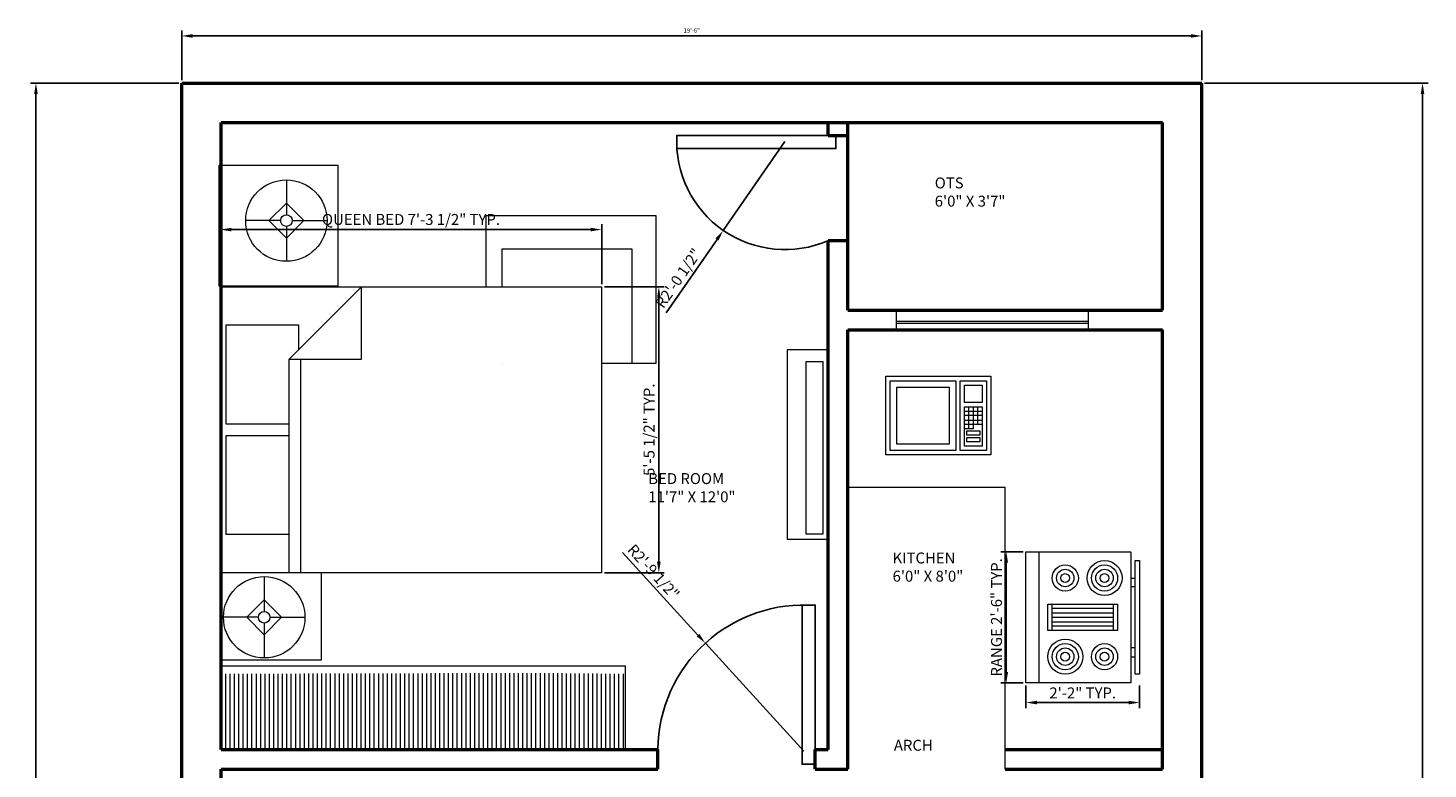
# Model space of a CAD drawing. Units: inches. Extents: x 210 to 950, y 0 to 561.
# Tile 3 of 5: x 228 to 548, y 382 to 551. Entities that reach past the tile are written whole.
import ezdxf

# ---------------------------------------------------------------- set-up
doc = ezdxf.new("R2010")
doc.units = ezdxf.units.IN
for name, color, linetype, lineweight in [('A-ANNO-DIMS', 2, 'Continuous', 18), ('A-ANNO-TEXT', 7, 'Continuous', 18), ('A-AREA-IDEN', 7, 'Continuous', 18), ('A-DOOR', 4, 'Continuous', 25), ('A-EQPM', 8, 'Continuous', 18), ('A-FLOR-CASE', 8, 'Continuous', 20), ('A-FURN', 8, 'Continuous', 18), ('A-FURN-PATT', 9, 'Continuous', 13), ('A-GLAZ', 4, 'Continuous', 20), ('A-WALL', 7, 'Continuous', 50)]:
    doc.layers.add(name, color=color, linetype=linetype, lineweight=lineweight)
doc.styles.get("Standard").update_dxf_attribs({"font": 'arial.ttf'})
doc.dimstyles.new('ISO-25', dxfattribs={"dimtxt": 2.5, "dimasz": 2.5, "dimexe": 1.25, "dimexo": 0.625, "dimtad": 1, "dimtxsty": 'Standard', "dimcen": 2.5, "dimadec": 0, "dimazin": 0, "dimtfac": 1, "dimtmove": 0, "dimatfit": 3, "dimfxl": 1, "dimarcsym": 0})

# ---------------------------------------------------------------- blocks, each defined once
blk = doc.blocks.new('Bed - Queen')
for p, q in [((0, -80.00003), (0, 0)), ((0, 0), (59.99999, 0)), ((59.99999, 0), (59.99999, -80.00003)), ((7.99999, -1.2), (28.79998, -1.2)), ((7.99999, -14.4), (7.99999, -1.2)), ((28.79998, -1.2), (28.79998, -14.4)), ((31.19999, -1.2), (51.99999, -1.2)), ((31.19999, -14.4), (31.19999, -1.2)), ((51.99999, -1.2), (51.99999, -16.4)), ((0, -14.4), (44.8, -14.4)), ((59.99999, -29.6), (44.8, -14.4)), ((44.8, -14.4), (44.8, -29.6)), ((44.8, -16.8), (0, -16.8)), ((51.99999, -16.4), (46.79936, -16.4)), ((44.8, -29.6), (59.99999, -29.6)), ((59.99999, -80.00003), (0, -80.00003))]:
    blk.add_line(p, q)
blk = doc.blocks.new('Lamp - Table')
for p, q in [((0, 7), (0, 1)), ((0, 3), (-3, 0)), ((3, 0), (0, 3)), ((-1, 0), (-7, 0)), ((-3, 0), (0, -3)), ((0, -3), (3, 0)), ((1, 0), (7, 0)), ((0, -1), (0, -7))]:
    blk.add_line(p, q)
for radius in [7, 1]:
    blk.add_circle((0, 0), radius)
blk = doc.blocks.new('Range-Oven - 30 in top')
for p, q in [((0, -3), (30, -3)), ((12, -6), (18, -6)), ((13, -20), (13, -6)), ((14, -6), (14, -20)), ((15, -20), (15, -6)), ((16, -6), (16, -20)), ((17, -20), (17, -6)), ((18, -20), (12, -20)), ((6, -24), (6, -25)), ((8, -25), (8, -24)), ((22, -25), (22, -24)), ((24, -24), (24, -25))]:
    blk.add_line(p, q)
for points in [[(0, -24), (0, 0), (30, 0), (30, -24)], [(12, -21), (12, -5), (18, -5), (18, -21)], [(2, -26), (2, -25), (28, -25), (28, -26)]]:
    blk.add_lwpolyline(points, close=True)
for centre, radius in [((6, -9), 4), ((6, -9), 3), ((24, -9), 3), ((6, -9), 2), ((6, -9), 1), ((24, -9), 2), ((24, -9), 1), ((6, -18), 3), ((6, -18), 2), ((24, -18), 4), ((24, -18), 3), ((24, -18), 2), ((6, -18), 1), ((24, -18), 1)]:
    blk.add_circle(centre, radius)
blk = doc.blocks.new('Microwave')
for p, q in [((18, 10), (22, 10)), ((19, 7), (19, 11)), ((20, 11), (20, 7)), ((21, 7), (21, 11)), ((22, 9), (18, 9)), ((18, 8), (22, 8)), ((22, 7), (18, 7)), ((19, 6), (19, 7)), ((20, 7), (20, 6)), ((20, 6), (18, 6))]:
    blk.add_line(p, q)
for points in [[(0, 0), (0, 18), (24, 18), (24, 0)], [(1, 1), (1, 17), (16, 17), (16, 1)], [(17, 1), (17, 17), (23, 17), (23, 1)], [(2.5, 2.5), (2.5, 15.5), (14.5, 15.5), (14.5, 2.5)], [(18, 12), (18, 16), (22, 16), (22, 12)], [(18, 2), (18, 11), (22, 11), (22, 2)], [(18.5, 4.5), (18.5, 5.5), (21.5, 5.5), (21.5, 4.5)], [(18.5, 3), (18.5, 4), (21.5, 4), (21.5, 3)]]:
    blk.add_lwpolyline(points, close=True)
blk = doc.blocks.new('*D14')
at = {"layer": 'A-ANNO-DIMS', "color": 0, "lineweight": -2, "transparency": 16777216}
for p, q in [((262.91, 539.13), (262.91, 550.53)), ((265.41, 549.28), (493.91, 549.28)), ((496.41, 539.13), (496.41, 550.53))]:
    blk.add_line(p, q, dxfattribs=at)
at = {"layer": 'A-ANNO-DIMS', "color": 0, "transparency": 16777216}
for points in [[(265.41, 549.7), (265.41, 548.87), (262.91, 549.28)], [(493.91, 549.7), (493.91, 548.87), (496.41, 549.28)]]:
    blk.add_solid(points, dxfattribs=at)
at = {"layer": 'Defpoints', "color": 0, "transparency": 16777216}
for p in [(496.41, 549.28), (262.91, 538.5), (496.41, 538.5)]:
    blk.add_point(p, dxfattribs=at)
at = {"layer": 'A-ANNO-DIMS', "color": 0, "transparency": 16777216, "insert": (379.66, 550.42), "char_height": 1, "attachment_point": 5}
blk.add_mtext('19\'-6"', dxfattribs=at)
blk = doc.blocks.new('*D15')
at = {"layer": 'A-ANNO-DIMS', "color": 0, "lineweight": -2, "transparency": 16777216}
for p, q in [((262.29, 538.5), (228.3, 538.5)), ((229.55, 61), (229.55, 536)), ((262.29, 58.5), (228.3, 58.5))]:
    blk.add_line(p, q, dxfattribs=at)
at = {"layer": 'A-ANNO-DIMS', "color": 0, "transparency": 16777216}
for points in [[(229.13, 536), (229.96, 536), (229.55, 538.5)], [(229.13, 61), (229.96, 61), (229.55, 58.5)]]:
    blk.add_solid(points, dxfattribs=at)
at = {"layer": 'Defpoints', "color": 0, "transparency": 16777216}
for p in [(229.55, 538.5), (262.91, 538.5), (262.91, 58.5)]:
    blk.add_point(p, dxfattribs=at)
at = {"layer": 'A-ANNO-DIMS', "color": 0, "transparency": 16777216, "insert": (228.41, 298.5), "char_height": 1, "attachment_point": 5, "rotation": 90}
blk.add_mtext("40'", dxfattribs=at)
blk = doc.blocks.new('*D16')
at = {"layer": 'A-ANNO-DIMS', "color": 0, "lineweight": -2, "transparency": 16777216}
for p, q in [((497.04, 538.5), (548.19, 538.5)), ((546.94, 57), (546.94, 536)), ((497.04, 54.5), (548.19, 54.5))]:
    blk.add_line(p, q, dxfattribs=at)
at = {"layer": 'A-ANNO-DIMS', "color": 0, "transparency": 16777216}
for points in [[(546.52, 536), (547.35, 536), (546.94, 538.5)], [(546.52, 57), (547.35, 57), (546.94, 54.5)]]:
    blk.add_solid(points, dxfattribs=at)
at = {"layer": 'Defpoints', "color": 0, "transparency": 16777216}
for p in [(496.41, 538.5), (546.94, 538.5), (496.41, 54.5)]:
    blk.add_point(p, dxfattribs=at)
at = {"layer": 'A-ANNO-DIMS', "color": 0, "transparency": 16777216, "insert": (545.8, 296.5), "char_height": 1, "attachment_point": 5, "rotation": 90}
blk.add_mtext('40\'-4"', dxfattribs=at)
blk = doc.blocks.new('DOOR-LEAF-36IN')
blk.add_lwpolyline([(0, 0), (0, -2.99), (-36.41, -2.99), (-36.41, 0)], close=True)
blk = doc.blocks.new('*D30')
at = {"layer": 'A-ANNO-DIMS', "color": 0, "lineweight": -2, "transparency": 16777216}
for p, q in [((271.77, 492.5), (271.77, 506.21)), ((356.54, 504.96), (274.27, 504.96)), ((359.04, 492.5), (359.04, 506.21))]:
    blk.add_line(p, q, dxfattribs=at)
at = {"layer": 'A-ANNO-DIMS', "color": 0, "transparency": 16777216}
for points in [[(274.27, 505.38), (274.27, 504.55), (271.77, 504.96)], [(356.54, 505.38), (356.54, 504.55), (359.04, 504.96)]]:
    blk.add_solid(points, dxfattribs=at)
at = {"layer": 'Defpoints', "color": 0, "transparency": 16777216}
for p in [(271.77, 504.96), (271.77, 491.87), (359.04, 491.87)]:
    blk.add_point(p, dxfattribs=at)
at = {"layer": 'A-ANNO-DIMS', "color": 0, "transparency": 16777216, "insert": (315.4, 506.96), "char_height": 2.5, "attachment_point": 5}
blk.add_mtext('QUEEN BED 7\'-3 1/2" TYP.', dxfattribs=at)
blk = doc.blocks.new('*D31')
at = {"layer": 'A-ANNO-DIMS', "color": 0, "lineweight": -2, "transparency": 16777216}
for p, q in [((359.66, 491.87), (373.38, 491.87)), ((372.13, 428.92), (372.13, 489.37)), ((359.66, 426.42), (373.38, 426.42))]:
    blk.add_line(p, q, dxfattribs=at)
at = {"layer": 'A-ANNO-DIMS', "color": 0, "transparency": 16777216}
for points in [[(371.71, 489.37), (372.54, 489.37), (372.13, 491.87)], [(371.71, 428.92), (372.54, 428.92), (372.13, 426.42)]]:
    blk.add_solid(points, dxfattribs=at)
at = {"layer": 'Defpoints', "color": 0, "transparency": 16777216}
for p in [(359.04, 491.87), (372.13, 491.87), (359.04, 426.42)]:
    blk.add_point(p, dxfattribs=at)
at = {"layer": 'A-ANNO-DIMS', "color": 0, "transparency": 16777216, "insert": (370.21, 459.15), "char_height": 2.5, "attachment_point": 5, "rotation": 90}
blk.add_mtext('5\'-5 1/2" TYP.', dxfattribs=at)
blk = doc.blocks.new('*D36')
at = {"layer": 'A-ANNO-DIMS', "color": 0, "lineweight": -2, "transparency": 16777216}
for p, q in [((455.53, 431.21), (450.4, 431.21)), ((451.65, 403.71), (451.65, 428.71)), ((455.53, 401.21), (450.4, 401.21))]:
    blk.add_line(p, q, dxfattribs=at)
at = {"layer": 'A-ANNO-DIMS', "color": 0, "transparency": 16777216}
for points in [[(451.24, 428.71), (452.07, 428.71), (451.65, 431.21)], [(451.24, 403.71), (452.07, 403.71), (451.65, 401.21)]]:
    blk.add_solid(points, dxfattribs=at)
at = {"layer": 'Defpoints', "color": 0, "transparency": 16777216}
for p in [(451.65, 431.21), (456.15, 431.21), (456.15, 401.21)]:
    blk.add_point(p, dxfattribs=at)
at = {"layer": 'A-ANNO-DIMS', "color": 0, "transparency": 16777216, "insert": (449.74, 416.21), "char_height": 2.5, "attachment_point": 5, "rotation": 90}
blk.add_mtext('RANGE 2\'-6" TYP.', dxfattribs=at)
blk = doc.blocks.new('*D37')
at = {"layer": 'A-ANNO-DIMS', "color": 0, "lineweight": -2, "transparency": 16777216}
for p, q in [((456.15, 400.58), (456.15, 395.46)), ((482.15, 400.58), (482.15, 395.46)), ((479.65, 396.71), (458.65, 396.71))]:
    blk.add_line(p, q, dxfattribs=at)
at = {"layer": 'A-ANNO-DIMS', "color": 0, "transparency": 16777216}
for points in [[(458.65, 397.13), (458.65, 396.29), (456.15, 396.71)], [(479.65, 397.13), (479.65, 396.29), (482.15, 396.71)]]:
    blk.add_solid(points, dxfattribs=at)
at = {"layer": 'Defpoints', "color": 0, "transparency": 16777216}
for p in [(456.15, 401.21), (482.15, 401.21), (456.15, 396.71)]:
    blk.add_point(p, dxfattribs=at)
at = {"layer": 'A-ANNO-DIMS', "color": 0, "transparency": 16777216, "insert": (469.15, 398.59), "char_height": 2.5, "attachment_point": 5}
blk.add_mtext('2\'-2" TYP.', dxfattribs=at)
blk = doc.blocks.new('*D53')
at = {"layer": 'A-ANNO-DIMS', "color": 0, "lineweight": -2, "transparency": 16777216}
for p, q in [((363.83, 431.06), (381.09, 412.15)), ((405.29, 385.62), (382.77, 410.3))]:
    blk.add_line(p, q, dxfattribs=at)
at = {"layer": 'A-ANNO-DIMS', "color": 0, "transparency": 16777216}
blk.add_solid([(381.4, 412.43), (380.78, 411.87), (382.77, 410.3)], dxfattribs=at)
at = {"layer": 'Defpoints', "color": 0, "transparency": 16777216}
for p in [(382.77, 410.3), (405.29, 385.62)]:
    blk.add_point(p, dxfattribs=at)
at = {"layer": 'A-ANNO-DIMS', "color": 0, "transparency": 16777216, "insert": (370.68, 426.4), "char_height": 2.5, "attachment_point": 5, "rotation": 312.3709}
blk.add_mtext('R2\'-9 1/2"', dxfattribs=at)
blk = doc.blocks.new('*D54')
at = {"layer": 'A-ANNO-DIMS', "color": 0, "lineweight": -2, "transparency": 16777216}
for p, q in [((400.96, 525.12), (386.87, 504.77)), ((373.83, 485.94), (385.45, 502.72))]:
    blk.add_line(p, q, dxfattribs=at)
at = {"layer": 'A-ANNO-DIMS', "color": 0, "transparency": 16777216}
blk.add_solid([(385.1, 502.96), (385.79, 502.48), (386.87, 504.77)], dxfattribs=at)
at = {"layer": 'Defpoints', "color": 0, "transparency": 16777216}
for p in [(400.96, 525.12), (386.87, 504.77)]:
    blk.add_point(p, dxfattribs=at)
at = {"layer": 'A-ANNO-DIMS', "color": 0, "transparency": 16777216, "insert": (376.84, 493.66), "char_height": 2.5, "attachment_point": 5, "rotation": 55.2977}
blk.add_mtext('R2\'-0 1/2"', dxfattribs=at)

msp = doc.modelspace()

# ---------------------------------------------------------------- hatches: boundary and pattern name
at = {"layer": 'A-FURN-PATT'}
h = msp.add_hatch(dxfattribs=at)
h.set_pattern_fill('ANSI31', color=256, scale=0.314961, angle=45, style=0)
h.paths.add_polyline_path([(271.97, 403.27), (271.97, 386.23), (297.62, 386.09), (322.62, 386.09), (364.47, 386.23), (364.47, 403.27), (348.68, 403.41), (323.68, 403.41)])

# ---------------------------------------------------------------- linework, layer by layer
at = {"layer": 'A-DOOR'}
for centre, radius, start, end in [((400.96, 525.12), 24.75, 176.8495, 293.746), ((405.29, 385.62), 33.41, 85.4748, 179.2678)]:
    msp.add_arc(centre, radius, start, end, dxfattribs=at)
at = {"layer": 'A-FLOR-CASE'}
for p in [(415.41, 446), (451.41, 381.5)]:
    msp.add_line(p, (451.41, 446), dxfattribs=at)
msp.add_lwpolyline([(271.86, 386.06), (364.51, 386.06), (364.51, 405.03), (271.86, 405.03)], close=True, dxfattribs=at)
at = {"layer": 'A-FURN'}
for points in [[(271.48, 519.7), (298.62, 519.7), (298.62, 492), (271.48, 492)], [(410.86, 477.41), (401.51, 477.41), (401.51, 434.14), (410.86, 434.14)], [(409.73, 474.7), (405.8, 474.7), (405.8, 435.33), (409.73, 435.33)], [(271.87, 426.46), (294.85, 426.46), (294.85, 406.39), (271.87, 406.39)]]:
    msp.add_lwpolyline(points, close=True, dxfattribs=at)
for points in [[(332.57, 491.87), (332.57, 508.16), (371.47, 508.16), (371.47, 474.33), (359.04, 474.33)], [(336.27, 491.87), (336.27, 500.53), (365.95, 500.53), (365.95, 474.28), (359.04, 474.28)], [(336.27, 474.28), (336.27, 474.33)]]:
    msp.add_lwpolyline(points, dxfattribs=at)
at = {"layer": 'A-GLAZ'}
for p, q in [((426.49, 482), (426.49, 486.5)), ((426.49, 486.5), (470.39, 486.5)), ((426.49, 484), (470.39, 484)), ((470.39, 486.5), (470.39, 482)), ((470.39, 483.5), (426.49, 483.5))]:
    msp.add_line(p, q, dxfattribs=at)
at = {"layer": 'A-WALL'}
for p, q in [((262.91, 54.5), (262.91, 538.5)), ((262.91, 538.5), (496.41, 538.5)), ((496.41, 54.5), (496.41, 538.5)), ((271.91, 529.5), (410.91, 529.5)), ((271.91, 386), (271.91, 529.5)), ((410.91, 529.5), (487.41, 529.5)), ((410.91, 526.5), (410.91, 529.5)), ((415.41, 526.5), (415.41, 529.5)), ((487.41, 486.5), (487.41, 529.5)), ((487.41, 486.5), (487.41, 529.5)), ((410.91, 526.5), (415.41, 526.5)), ((415.41, 486.5), (415.41, 526.5)), ((410.91, 386), (410.91, 502.5)), ((410.91, 502.5), (415.41, 502.5)), ((415.41, 486.5), (487.41, 486.5)), ((415.41, 381.5), (415.41, 482)), ((415.41, 482), (487.41, 482)), ((487.41, 381.5), (487.41, 482)), ((487.41, 386), (487.41, 482)), ((271.91, 386), (371.91, 386)), ((371.91, 381.5), (371.91, 386)), ((407.91, 381.5), (407.91, 386)), ((407.91, 386), (410.91, 386)), ((451.41, 386), (487.41, 386)), ((271.91, 381.5), (371.91, 381.5)), ((271.91, 249.5), (271.91, 381.5)), ((407.91, 381.5), (415.41, 381.5)), ((451.41, 381.5), (487.41, 381.5))]:
    msp.add_line(p, q, dxfattribs=at)

# ---------------------------------------------------------------- block references
at = {"layer": 'A-DOOR'}
msp.add_blockref('DOOR-LEAF-36IN', (412.67, 526.5), dxfattribs=at)
at = {"layer": 'A-DOOR', "rotation": 270}
msp.add_blockref('DOOR-LEAF-36IN', (407.92, 382.6), dxfattribs=at)
at = {"layer": 'A-EQPM'}
msp.add_blockref('Microwave', (424.11, 453.38), dxfattribs=at)
at = {"layer": 'A-EQPM', "rotation": 90}
msp.add_blockref('Range-Oven - 30 in top', (456.15, 401.21), dxfattribs=at)
at = {"layer": 'A-FURN', "xscale": 1.330786106251803, "yscale": 1.330786106251803, "zscale": 1.330786106251803}
for p in [(286.87, 507.02), (281.79, 416.23)]:
    msp.add_blockref('Lamp - Table', p, dxfattribs=at)
at = {"layer": 'A-FURN', "xscale": 1.090825566177695, "yscale": 1.090825566177695, "zscale": 1.090825566177695, "rotation": 90}
msp.add_blockref('Bed - Queen', (271.77, 426.42), dxfattribs=at)

# ---------------------------------------------------------------- texts
at = {"layer": 'A-ANNO-TEXT', "insert": (425.93, 388.18), "char_height": 2.5, "attachment_point": 1}
msp.add_mtext_dynamic_manual_height_columns('ARCH', width=6.915, gutter_width=12.5, heights=[0], dxfattribs=at)
at = {"layer": 'A-AREA-IDEN', "char_height": 2.5, "attachment_point": 1}
for s, width, insert in [('OTS\\P6\'0" X 3\'7"', 23.4882, (435.28, 516.89)), ('BED ROOM\\P11\'7" X 12\'0"', 30.419, (369.71, 449.22)), ('KITCHEN\\P\\pxt5;6\'0" X 8\'0"', 25.4662, (425.63, 431.05))]:
    msp.add_mtext_dynamic_manual_height_columns(s, width=width, gutter_width=12.5, heights=[0], dxfattribs=dict(at, insert=insert))

# ---------------------------------------------------------------- dimensions: what is measured, and where the dimension line sits
at = {"layer": 'A-ANNO-DIMS'}
dim = msp.add_linear_dim(base=(496.41085496, 549.28267643), p1=(262.91085496, 538.50240855), p2=(496.41085496, 538.50240855), dimstyle='ISO-25', override={"dimtxt": 1, "dimdec": 0, "dimlunit": 3, "dimclrd": 0, "dimclre": 0, "dimclrt": 0, "dimtdec": 0}, dxfattribs=at)
dim.commit()
dim.dimension.update_dxf_attribs({"geometry": '*D14', "text_midpoint": (379.66085496, 550.41824942)})
for base, p1, p2, picture, middle in [((229.55, 538.5), (262.91, 58.5), (262.91, 538.5), '*D15', (228.41, 298.5)), ((546.94, 538.5), (496.41, 54.5), (496.41, 538.5), '*D16', (545.8, 296.5))]:
    dim = msp.add_linear_dim(base=base, p1=p1, p2=p2, angle=90, dimstyle='ISO-25', override={"dimtxt": 1, "dimdec": 0, "dimlunit": 3, "dimclrd": 0, "dimclre": 0, "dimclrt": 0, "dimtdec": 0}, dxfattribs=at)
    dim.commit()
    dim.dimension.update_dxf_attribs({"geometry": picture, "text_midpoint": middle})
for center, mpoint, picture, middle in [((400.9582, 525.1201), (386.8683, 504.7734), '*D54', (378.4144, 492.5654)), ((405.29, 385.62), (382.77, 410.3), '*D53', (369.26, 425.11))]:
    dim = msp.add_radius_dim(center=center, mpoint=mpoint, dimstyle='ISO-25', override={"dimdec": 1, "dimlfac": 1, "dimrnd": 0, "dimzin": 1, "dimdsep": 46, "dimlunit": 4, "dimfrac": 2}, dxfattribs=at)
    dim.commit()
    dim.dimension.update_dxf_attribs({"geometry": picture, "text_midpoint": middle, "dimtype": 164})
for base, p1, p2, angle, text, picture, middle in [((271.77, 504.96), (359.04, 491.87), (271.77, 491.87), 180, 'QUEEN BED <> TYP.', '*D30', (315.4, 506.96)), ((372.1274, 491.8735), (359.0375, 426.424), (359.0375, 491.8735), 90, '<> TYP.', '*D31', (370.2097, 459.1488)), ((451.65, 431.21), (456.15, 401.21), (456.15, 431.21), 90, 'RANGE <> TYP.', '*D36', (449.74, 416.21)), ((456.15, 396.71), (482.15, 401.21), (456.15, 401.21), 180, '<> TYP.', '*D37', (469.15, 398.59))]:
    dim = msp.add_linear_dim(base=base, p1=p1, p2=p2, angle=angle, text=text, dimstyle='ISO-25', override={"dimdec": 1, "dimlfac": 1, "dimrnd": 0, "dimzin": 1, "dimdsep": 46, "dimlunit": 4, "dimfrac": 2}, dxfattribs=at)
    dim.commit()
    dim.dimension.update_dxf_attribs({"geometry": picture, "text_midpoint": middle})

doc.saveas('drawing.dxf')
